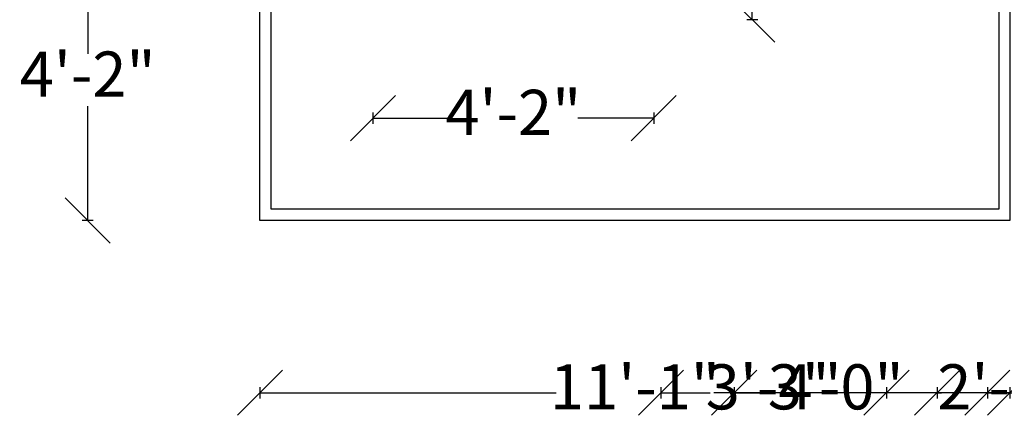
# Model space of a CAD drawing. Units: inches. Extents: x 3121 to 3511, y 1323 to 1998.
# Tile 1 of 10: x 3147 to 3322, y 1330 to 1402. Entities that reach past the tile are written whole.
import ezdxf

# ---------------------------------------------------------------- set-up
doc = ezdxf.new("R2010")
doc.units = ezdxf.units.IN
doc.layers.add('A-ANNO-DIMS', color=2, linetype='Continuous', lineweight=18)
doc.layers.add('A-FLOR', color=7, linetype='Continuous', lineweight=25)
doc.styles.get("Standard").update_dxf_attribs({"font": 'arial.ttf'})
doc.dimstyles.new('ISO-25', dxfattribs={"dimtxt": 8, "dimasz": 8, "dimexe": 1, "dimexo": 1, "dimtad": 0, "dimtih": 1, "dimtoh": 1, "dimlunit": 3, "dimtxsty": 'Standard', "dimblk": 'OBLIQUE', "dimcen": 2.5, "dimclrt": 1, "dimadec": 0, "dimazin": 0, "dimtfac": 1, "dimtmove": 0, "dimatfit": 3, "dimfxl": 1, "dimfxlon": 1, "dimarcsym": 0})

# ---------------------------------------------------------------- blocks, each defined once
blk = doc.blocks.new('_Oblique')
at = {"color": 0, "linetype": 'ByBlock', "lineweight": -2}
blk.add_line((-0.5, -0.5), (0.5, 0.5), dxfattribs=at)
blk = doc.blocks.new('*D31')
at = {"layer": 'A-ANNO-DIMS', "color": 0, "lineweight": -2, "transparency": 16777216}
for p, q in [((3276.23, 1518.07), (3278.23, 1518.07)), ((3277.23, 1518.07), (3277.23, 1464.56)), ((3277.23, 1401.54), (3277.23, 1455.04)), ((3276.23, 1401.54), (3278.23, 1401.54))]:
    blk.add_line(p, q, dxfattribs=at)
at = {"layer": 'Defpoints', "color": 0, "transparency": 16777216}
for p in [(3259.75, 1518.07), (3277.23, 1518.07), (3259.75, 1401.54)]:
    blk.add_point(p, dxfattribs=at)
at = {"layer": 'A-ANNO-DIMS', "color": 0, "lineweight": -2, "transparency": 16777216, "xscale": 8, "yscale": 8, "zscale": 8}
for p, rotation in [((3277.23, 1518.07), 90), ((3277.23, 1401.54), 270)]:
    blk.add_blockref('_Oblique', p, dxfattribs=dict(at, rotation=rotation))
at = {"layer": 'A-ANNO-DIMS', "color": 1, "transparency": 16777216, "insert": (3277.23, 1459.8), "char_height": 8, "attachment_point": 5}
blk.add_mtext('CAR 9\'-8 1/2"', dxfattribs=at)
blk = doc.blocks.new('*D32')
at = {"layer": 'A-ANNO-DIMS', "color": 0, "lineweight": -2, "transparency": 16777216}
for p, q in [((3209.95, 1385.06), (3209.95, 1383.06)), ((3259.75, 1385.06), (3259.75, 1383.06)), ((3209.95, 1384.06), (3223.43, 1384.06)), ((3259.75, 1384.06), (3246.27, 1384.06))]:
    blk.add_line(p, q, dxfattribs=at)
at = {"layer": 'Defpoints', "color": 0, "transparency": 16777216}
for p in [(3209.95, 1401.54), (3259.75, 1401.54), (3259.75, 1384.06)]:
    blk.add_point(p, dxfattribs=at)
at = {"layer": 'A-ANNO-DIMS', "color": 0, "lineweight": -2, "transparency": 16777216, "xscale": 8, "yscale": 8, "zscale": 8, "rotation": 180}
blk.add_blockref('_Oblique', (3209.95, 1384.06), dxfattribs=at)
at = {"layer": 'A-ANNO-DIMS', "color": 0, "lineweight": -2, "transparency": 16777216, "xscale": 8, "yscale": 8, "zscale": 8}
blk.add_blockref('_Oblique', (3259.75, 1384.06), dxfattribs=at)
at = {"layer": 'A-ANNO-DIMS', "color": 1, "transparency": 16777216, "insert": (3234.85, 1384.06), "char_height": 8, "attachment_point": 5}
blk.add_mtext('4\'-2"', dxfattribs=at)
blk = doc.blocks.new('*D33')
at = {"layer": 'A-ANNO-DIMS', "color": 0, "lineweight": -2, "transparency": 16777216}
for p, q in [((3160.37, 1415.78), (3158.37, 1415.78)), ((3159.37, 1415.78), (3159.37, 1395.49)), ((3159.37, 1365.92), (3159.37, 1386.21)), ((3160.37, 1365.92), (3158.37, 1365.92))]:
    blk.add_line(p, q, dxfattribs=at)
at = {"layer": 'Defpoints', "color": 0, "transparency": 16777216}
for p in [(3159.37, 1415.78), (3189.92, 1415.78), (3189.92, 1365.92)]:
    blk.add_point(p, dxfattribs=at)
at = {"layer": 'A-ANNO-DIMS', "color": 0, "lineweight": -2, "transparency": 16777216, "xscale": 8, "yscale": 8, "zscale": 8}
for p, rotation in [((3159.37, 1415.78), 90), ((3159.37, 1365.92), 270)]:
    blk.add_blockref('_Oblique', p, dxfattribs=dict(at, rotation=rotation))
at = {"layer": 'A-ANNO-DIMS', "color": 1, "transparency": 16777216, "insert": (3159.37, 1390.85), "char_height": 8, "attachment_point": 5}
blk.add_mtext('4\'-2"', dxfattribs=at)
blk = doc.blocks.new('*D34')
at = {"layer": 'A-ANNO-DIMS', "color": 0, "lineweight": -2, "transparency": 16777216}
for p, q in [((3189.92, 1336.37), (3189.92, 1334.37)), ((3322.92, 1336.37), (3322.92, 1334.37)), ((3189.92, 1335.37), (3242.43, 1335.37)), ((3322.92, 1335.37), (3270.41, 1335.37))]:
    blk.add_line(p, q, dxfattribs=at)
at = {"layer": 'Defpoints', "color": 0, "transparency": 16777216}
for p in [(3189.92, 1365.92), (3322.92, 1365.92), (3322.92, 1335.37)]:
    blk.add_point(p, dxfattribs=at)
at = {"layer": 'A-ANNO-DIMS', "color": 0, "lineweight": -2, "transparency": 16777216, "xscale": 8, "yscale": 8, "zscale": 8, "rotation": 180}
blk.add_blockref('_Oblique', (3189.92, 1335.37), dxfattribs=at)
at = {"layer": 'A-ANNO-DIMS', "color": 0, "lineweight": -2, "transparency": 16777216, "xscale": 8, "yscale": 8, "zscale": 8}
blk.add_blockref('_Oblique', (3322.92, 1335.37), dxfattribs=at)
at = {"layer": 'A-ANNO-DIMS', "color": 1, "transparency": 16777216, "insert": (3256.42, 1335.37), "char_height": 8, "attachment_point": 5}
blk.add_mtext('11\'-1"', dxfattribs=at)
blk = doc.blocks.new('*D53')
at = {"layer": 'A-ANNO-DIMS', "color": 0, "lineweight": -2, "transparency": 16777216}
for p, q in [((3274.02, 1336.37), (3274.02, 1334.37)), ((3310.02, 1336.37), (3310.02, 1334.37)), ((3274.02, 1335.37), (3280.77, 1335.37)), ((3310.02, 1335.37), (3303.28, 1335.37))]:
    blk.add_line(p, q, dxfattribs=at)
at = {"layer": 'Defpoints', "color": 0, "transparency": 16777216}
for p in [(3274.02, 1946.78), (3310.02, 1946.78), (3310.02, 1335.37)]:
    blk.add_point(p, dxfattribs=at)
at = {"layer": 'A-ANNO-DIMS', "color": 0, "lineweight": -2, "transparency": 16777216, "xscale": 8, "yscale": 8, "zscale": 8, "rotation": 180}
blk.add_blockref('_Oblique', (3274.02, 1335.37), dxfattribs=at)
at = {"layer": 'A-ANNO-DIMS', "color": 0, "lineweight": -2, "transparency": 16777216, "xscale": 8, "yscale": 8, "zscale": 8}
blk.add_blockref('_Oblique', (3310.02, 1335.37), dxfattribs=at)
at = {"layer": 'A-ANNO-DIMS', "color": 1, "transparency": 16777216, "insert": (3292.02, 1335.37), "char_height": 8, "attachment_point": 5}
blk.add_mtext('3\'-0"', dxfattribs=at)
blk = doc.blocks.new('*D54')
at = {"layer": 'A-ANNO-DIMS', "color": 0, "lineweight": -2, "transparency": 16777216}
for p, q in [((3310.02, 1336.37), (3310.02, 1334.37)), ((3334.16, 1336.37), (3334.16, 1334.37)), ((3310.02, 1335.37), (3310.76, 1335.37)), ((3334.16, 1335.37), (3333.42, 1335.37))]:
    blk.add_line(p, q, dxfattribs=at)
at = {"layer": 'Defpoints', "color": 0, "transparency": 16777216}
for p in [(3310.02, 1946.78), (3334.16, 1946.78), (3334.16, 1335.37)]:
    blk.add_point(p, dxfattribs=at)
at = {"layer": 'A-ANNO-DIMS', "color": 0, "lineweight": -2, "transparency": 16777216, "xscale": 8, "yscale": 8, "zscale": 8, "rotation": 180}
blk.add_blockref('_Oblique', (3310.02, 1335.37), dxfattribs=at)
at = {"layer": 'A-ANNO-DIMS', "color": 0, "lineweight": -2, "transparency": 16777216, "xscale": 8, "yscale": 8, "zscale": 8}
blk.add_blockref('_Oblique', (3334.16, 1335.37), dxfattribs=at)
at = {"layer": 'A-ANNO-DIMS', "color": 1, "transparency": 16777216, "insert": (3322.09, 1335.37), "char_height": 8, "attachment_point": 5}
blk.add_mtext('2\'-0"', dxfattribs=at)
blk = doc.blocks.new('*D59')
at = {"layer": 'A-ANNO-DIMS', "color": 0, "lineweight": -2, "transparency": 16777216}
for p, q in [((3318.92, 1336.37), (3318.92, 1334.37)), ((3370.92, 1336.37), (3370.92, 1334.37)), ((3318.92, 1335.37), (3333.5, 1335.37)), ((3370.92, 1335.37), (3356.34, 1335.37))]:
    blk.add_line(p, q, dxfattribs=at)
at = {"layer": 'Defpoints', "color": 0, "transparency": 16777216}
for p in [(3318.92, 1752.23), (3370.92, 1748.78), (3370.92, 1335.37)]:
    blk.add_point(p, dxfattribs=at)
at = {"layer": 'A-ANNO-DIMS', "color": 0, "lineweight": -2, "transparency": 16777216, "xscale": 8, "yscale": 8, "zscale": 8, "rotation": 180}
blk.add_blockref('_Oblique', (3318.92, 1335.37), dxfattribs=at)
at = {"layer": 'A-ANNO-DIMS', "color": 0, "lineweight": -2, "transparency": 16777216, "xscale": 8, "yscale": 8, "zscale": 8}
blk.add_blockref('_Oblique', (3370.92, 1335.37), dxfattribs=at)
at = {"layer": 'A-ANNO-DIMS', "color": 1, "transparency": 16777216, "insert": (3344.92, 1335.37), "char_height": 8, "attachment_point": 5}
blk.add_mtext('4\'-4"', dxfattribs=at)
blk = doc.blocks.new('*D73')
at = {"layer": 'A-ANNO-DIMS', "color": 0, "lineweight": -2, "transparency": 16777216}
for p, q in [((3261.02, 1336.37), (3261.02, 1334.37)), ((3301.03, 1336.37), (3301.03, 1334.37)), ((3261.02, 1335.37), (3269.77, 1335.37)), ((3301.03, 1335.37), (3292.28, 1335.37))]:
    blk.add_line(p, q, dxfattribs=at)
at = {"layer": 'Defpoints', "color": 0, "transparency": 16777216}
for p in [(3261.02, 1739.78), (3301.03, 1739.78), (3301.03, 1335.37)]:
    blk.add_point(p, dxfattribs=at)
at = {"layer": 'A-ANNO-DIMS', "color": 0, "lineweight": -2, "transparency": 16777216, "xscale": 8, "yscale": 8, "zscale": 8, "rotation": 180}
blk.add_blockref('_Oblique', (3261.02, 1335.37), dxfattribs=at)
at = {"layer": 'A-ANNO-DIMS', "color": 0, "lineweight": -2, "transparency": 16777216, "xscale": 8, "yscale": 8, "zscale": 8}
blk.add_blockref('_Oblique', (3301.03, 1335.37), dxfattribs=at)
at = {"layer": 'A-ANNO-DIMS', "color": 1, "transparency": 16777216, "insert": (3281.02, 1335.37), "char_height": 8, "attachment_point": 5}
blk.add_mtext('3\'-4"', dxfattribs=at)

msp = doc.modelspace()

# ---------------------------------------------------------------- linework, layer by layer
at = {"layer": 'A-FLOR'}
for points in [[(3322.918, 1415.784), (3322.918, 1365.917), (3189.918, 1365.917), (3189.918, 1415.784)], [(3320.918, 1415.784), (3320.918, 1367.917), (3191.918, 1367.917), (3191.918, 1415.784)]]:
    msp.add_lwpolyline(points, dxfattribs=at)

# ---------------------------------------------------------------- dimensions: what is measured, and where the dimension line sits
at = {"layer": 'A-ANNO-DIMS'}
for base, p1, p2, picture, middle in [((3310.023, 1335.367), (3274.023, 1946.784), (3310.023, 1946.784), '*D53', (3292.023, 1335.367)), ((3334.156, 1335.367), (3310.023, 1946.784), (3334.156, 1946.784), '*D54', (3322.089, 1335.367)), ((3370.918, 1335.367), (3318.918, 1752.226), (3370.918, 1748.784), '*D59', (3344.918, 1335.367)), ((3301.026, 1335.367), (3261.023, 1739.784), (3301.026, 1739.784), '*D73', (3281.024, 1335.367)), ((3259.751, 1384.055), (3209.949, 1401.535), (3259.751, 1401.535), '*D32', (3234.85, 1384.055)), ((3322.918, 1335.367), (3189.918, 1365.917), (3322.918, 1365.917), '*D34', (3256.418, 1335.367))]:
    dim = msp.add_linear_dim(base=base, p1=p1, p2=p2, dimstyle='ISO-25', override={"dimdec": 1, "dimlfac": 1, "dimrnd": 0, "dimzin": 1, "dimdsep": 46, "dimlunit": 4, "dimfrac": 2}, dxfattribs=at)
    dim.commit()
    dim.dimension.update_dxf_attribs({"geometry": picture, "text_midpoint": middle})
dim = msp.add_linear_dim(base=(3277.231, 1518.068), p1=(3259.751, 1401.535), p2=(3259.751, 1518.068), angle=90, text='CAR <>', dimstyle='ISO-25', override={"dimdec": 1, "dimlfac": 1, "dimrnd": 0, "dimzin": 1, "dimdsep": 46, "dimlunit": 4, "dimfrac": 2}, dxfattribs=at)
dim.commit()
dim.dimension.update_dxf_attribs({"geometry": '*D31', "text_midpoint": (3277.231, 1459.801)})
dim = msp.add_linear_dim(base=(3159.368, 1415.784), p1=(3189.918, 1365.917), p2=(3189.918, 1415.784), angle=90, dimstyle='ISO-25', override={"dimdec": 1, "dimlfac": 1, "dimrnd": 0, "dimzin": 1, "dimdsep": 46, "dimlunit": 4, "dimfrac": 2}, dxfattribs=at)
dim.commit()
dim.dimension.update_dxf_attribs({"geometry": '*D33', "text_midpoint": (3159.368, 1390.851)})

doc.saveas('drawing.dxf')
